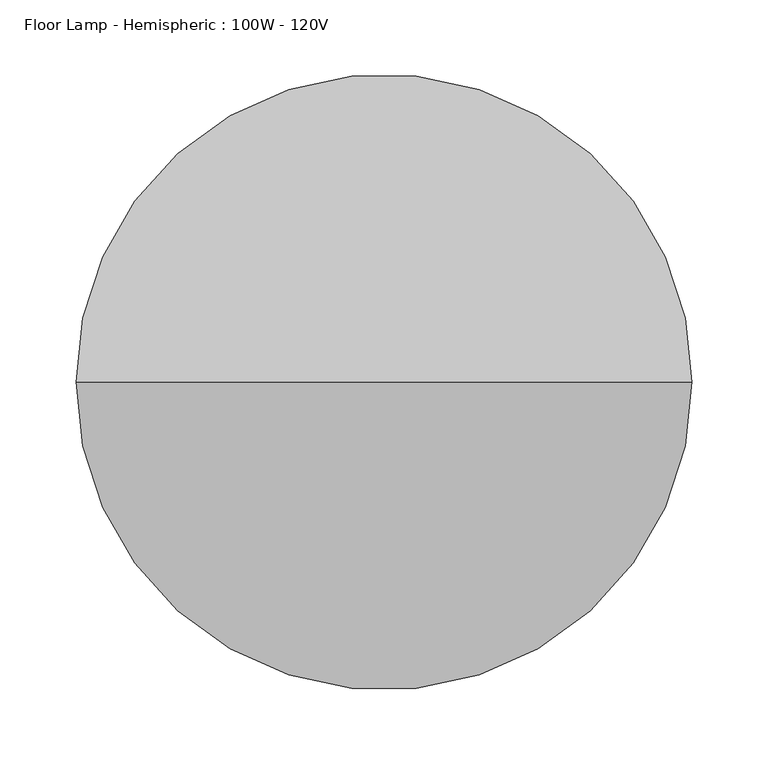
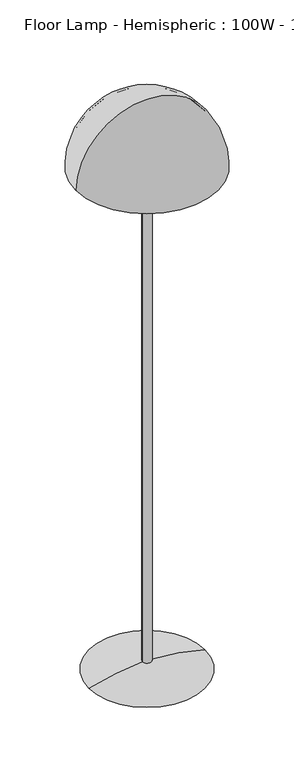
"""IFC4 building model written with IfcOpenShell, lengths in millimetres: light fixture geometry, Floor Lamp - Hemispheric : 100W - 120V."""

from ifc_helpers import new_model, si_unit, point, frame, origin, origin_with_axes, origin_2d, place, context, project, spatial, polyline, circle_curve, ellipse_curve, trimmed, segment, composite_curve, outline, extrude, source, transform, mapped, element, save
from ifc_brep_helpers import plane_surface, revolved_surface, advanced_brep


def floor_lamp_hemispheric_100w_120v_bd9db648(model_context):
    return source(origin(), model_context, "Body", "SolidModel", [
        advanced_brep(
        [(-197.591573, 0.0, 1510.4133868), (197.591573, 0.0, 1510.4133868), (0.0, 0.0, 1707.4075084), (-202.3305676, 0.0, 1510.4133868), (202.3305676, 0.0, 1510.4133868), (0.0, 0.0, 1713.4837615)],
        [
            (0, 1, circle_curve(frame((0.0, 0.0, 1510.4133868), z_axis=(0.0, 0.0, -1.0), x_axis=(1.0, 0.0, 0.0)), 197.591573)),
            (1, 2, circle_curve(frame((0.7416268, 0.0, 1510.5589055), z_axis=(0.0, -1.0, 0.0), x_axis=(1.0, 0.0, 0.0)), 196.85)),
            (2, 0, circle_curve(frame((-0.7416268, 0.0, 1510.5589055), z_axis=(0.0, -1.0, 0.0), x_axis=(-1.0, 0.0, 0.0)), 196.85)),
            (1, 0, circle_curve(frame((0.0, 0.0, 1510.4133868), z_axis=(0.0, 0.0, -1.0), x_axis=(1.0, 0.0, 0.0)), 197.591573)),
            (3, 4, circle_curve(frame((0.0, 0.0, 1510.4133868), z_axis=(0.0, 0.0, -1.0), x_axis=(1.0, 0.0, 0.0)), 202.3305676)),
            (4, 1),
            (0, 3),
            (4, 3, circle_curve(frame((0.0, 0.0, 1510.4133868), z_axis=(0.0, 0.0, -1.0), x_axis=(1.0, 0.0, 0.0)), 202.3305676)),
            (5, 4, circle_curve(frame((-0.8693923, 0.0, 1510.2856214), z_axis=(0.0, 1.0, 0.0), x_axis=(1.0, 0.0, 0.0)), 203.2)),
            (3, 5, circle_curve(frame((0.8693923, 0.0, 1510.2856214), z_axis=(0.0, 1.0, 0.0), x_axis=(-1.0, 0.0, 0.0)), 203.2)),
        ],
        [
            revolved_surface(trimmed(ellipse_curve(frame((0.7416268, 0.0, 1510.5589055), z_axis=(0.0, 1.0, 0.0), x_axis=(1.0, 0.0, 0.0)), 196.85, 196.85), [point((0.0, 0.0, 1707.4075084))], [point((197.591573, 0.0, 1510.4133868))], True, "CARTESIAN"), (0.0, 0.0, 1815.2133868), (0.0, 0.0, 1.0)),
            plane_surface(frame((0.0, 0.0, 1510.4133868), z_axis=(0.0, 0.0, -1.0), x_axis=(1.0, 0.0, 0.0))),
            revolved_surface(trimmed(ellipse_curve(frame((-0.8693923, 0.0, 1510.2856214), z_axis=(0.0, -1.0, 0.0), x_axis=(1.0, 0.0, 0.0)), 203.2, 203.2), [point((202.3305676, 0.0, 1510.4133868))], [point((0.0, 0.0, 1713.4837615))], True, "CARTESIAN"), (0.0, 0.0, 1815.2133868), (0.0, 0.0, 1.0)),
        ],
        [
            (0, [[1, 2, 3]]),
            (0, [[4, -3, -2]]),
            (1, [[5, 6, -1, 7]]),
            (1, [[8, -7, -4, -6]]),
            (2, [[9, -5, 10]]),
            (2, [[-10, -8, -9]]),
        ],
    ),
        advanced_brep(
        [(-165.1, 0.0, 0.0), (165.1, 0.0, 0.0), (12.7, 0.0, 0.0), (-12.7, 0.0, 0.0), (-12.7, 0.0, 25.4), (12.7, 0.0, 25.4)],
        [
            (0, 1, circle_curve(frame((0.0, 0.0, 0.0), z_axis=(0.0, 0.0, -1.0), x_axis=(1.0, 0.0, 0.0)), 165.1)),
            (1, 2),
            (2, 3, circle_curve(origin_with_axes(), 12.7)),
            (3, 0),
            (1, 0, circle_curve(frame((0.0, 0.0, 0.0), z_axis=(0.0, 0.0, -1.0), x_axis=(1.0, 0.0, 0.0)), 165.1)),
            (3, 2, circle_curve(origin_with_axes(), 12.7)),
            (4, 5, circle_curve(frame((0.0, 0.0, 25.4), z_axis=(0.0, 0.0, -1.0), x_axis=(1.0, 0.0, 0.0)), 12.7)),
            (5, 1, circle_curve(frame((-10.5405788, 0.0, -583.9434729), z_axis=(0.0, 1.0, 0.0), x_axis=(1.0, 0.0, 0.0)), 609.7865138)),
            (0, 4, circle_curve(frame((10.5405788, 0.0, -583.9434729), z_axis=(0.0, 1.0, 0.0), x_axis=(-1.0, 0.0, 0.0)), 609.7865138)),
            (5, 4, circle_curve(frame((0.0, 0.0, 25.4), z_axis=(0.0, 0.0, -1.0), x_axis=(1.0, 0.0, 0.0)), 12.7)),
            (2, 5),
            (4, 3),
        ],
        [
            plane_surface(frame((0.0, 0.0, 0.0), z_axis=(0.0, 0.0, -1.0), x_axis=(1.0, 0.0, 0.0))),
            revolved_surface(trimmed(ellipse_curve(frame((-10.5405788, 0.0, -583.9434729), z_axis=(0.0, -1.0, 0.0), x_axis=(1.0, 0.0, 0.0)), 609.7865138, 609.7865138), [point((165.1, 0.0, 0.0))], [point((12.7, 0.0, 25.4))], True, "CARTESIAN"), (0.0, 0.0, 127.0), (0.0, 0.0, 1.0)),
            revolved_surface(polyline([(12.7, 0.0, 25.400000000000006), (12.7, 0.0, 0.0)]), (0.0, 0.0, 127.0), (0.0, 0.0, 1.0)),
        ],
        [
            (0, [[1, 2, 3, 4]]),
            (0, [[5, -4, 6, -2]]),
            (1, [[7, 8, -1, 9]]),
            (1, [[10, -9, -5, -8]]),
            (2, [[-3, 11, -7, 12]]),
            (2, [[-6, -12, -10, -11]]),
        ],
    ),
        extrude(outline(composite_curve([segment(trimmed(circle_curve(origin_2d(), 12.7), [point((-12.7, 0.0))], [point((12.7, 0.0))], False, "CARTESIAN"), True, "CONTINUOUS"), segment(trimmed(circle_curve(origin_2d(), 12.7), [point((12.7, 0.0))], [point((-12.7, 0.0))], False, "CARTESIAN"), True, "CONTINUOUS")], self_intersect=False)), frame((0.0, 0.0, 25.4), z_axis=(0.0, 0.0, 1.0), x_axis=(1.0, 0.0, 0.0)), (0.0, 0.0, 1.0), 1524.0),
    ])


if __name__ == "__main__":
    model = new_model("IFC4")
    model_context = context("Model", 3, world=origin())
    ifc_project = project(units=[si_unit("LENGTHUNIT", "METRE", prefix="MILLI")], contexts=[model_context])
    site = spatial("IfcSite", under=ifc_project)
    building = spatial("IfcBuilding", under=site)
    placement = place(None, origin())
    floor_lamp_hemispheric_100w_120v_shape = floor_lamp_hemispheric_100w_120v_bd9db648(model_context)
    element("IfcLightFixture", 1, ObjectType="Floor Lamp - Hemispheric : 100W - 120V", at=placement, inside=building, context=model_context, shape_type="MappedRepresentation", body=[
        mapped(floor_lamp_hemispheric_100w_120v_shape, transform((0.0, 0.0, 0.0), x_axis=(1.0, 0.0, 0.0), y_axis=(0.0, 1.0, 0.0), z_axis=(0.0, 0.0, 1.0))),
    ])
    save(model, "model.ifc")

# Revit data of these elements
# Type "Floor Lamp - Hemispheric : 100W - 120V"
#   Assembly Code = "D5020220"
#   Lamp = "A-19"
#   Wattage Comments = "100"
#   Wattage = 100 W
#   built-in parameter 1150110 = 1 (stored number, unit not read)
#   built-in parameter 1114217 = 1 (stored number, unit not read)
#   built-in parameter 1150109 = 1 (stored number, unit not read)
#   built-in parameter 1150113 = 1 (stored number, unit not read)
#   built-in parameter 1150115 = 1 (stored number, unit not read)
#   built-in parameter 1150105 = 557.042 (stored number, unit not read)
#   Light Source Symbol Size = 2' - 0"
#   built-in parameter 1150112 = 1 (stored number, unit not read)
#   built-in parameter 1150114 = 1 (stored number, unit not read)
#   built-in parameter 1150107 = 2800 (stored number, unit not read)
#   built-in parameter 1150106 = 5.57042 (stored number, unit not read)
#   built-in parameter 1150104 = 1.6258 (stored number, unit not read)
#   Ballast Voltage = 120 V
#   built-in parameter 1114218 = 1 (stored number, unit not read)
#   built-in parameter 1150133 = 10 (stored number, unit not read)
#   Lumens = 1750 lm
#   Apparent Load = 100 VA
#   built-in parameter 1150134 = 4
#   built-in parameter 1150137 = 1
#   Color Filter = 16777215
#   Ballast Number of Poles = 1
#   Shade = Glass, Frosted
#   Stand = Steel, Chrome Plated
#   Dimming Lamp Color Temperature Shift = (empty or 0)
#   Default Elevation = 0
# Element 1 (IfcLightFixture, "Floor Lamp - Hemispheric : 100W - 120V")
#   Materials on its faces: "Steel, Chrome Plated", "Glass, Frosted"
# Materials
#   "Glass, Frosted": class "Glass", colour RGB 250 244 225, transparency 0.55, Description = "physical material", Cost = 0
#   "Steel, Chrome Plated": class "Metal", colour RGB 17 17 17, transparency 0, Description = "Chromiuim plated steel", Cost = 0
